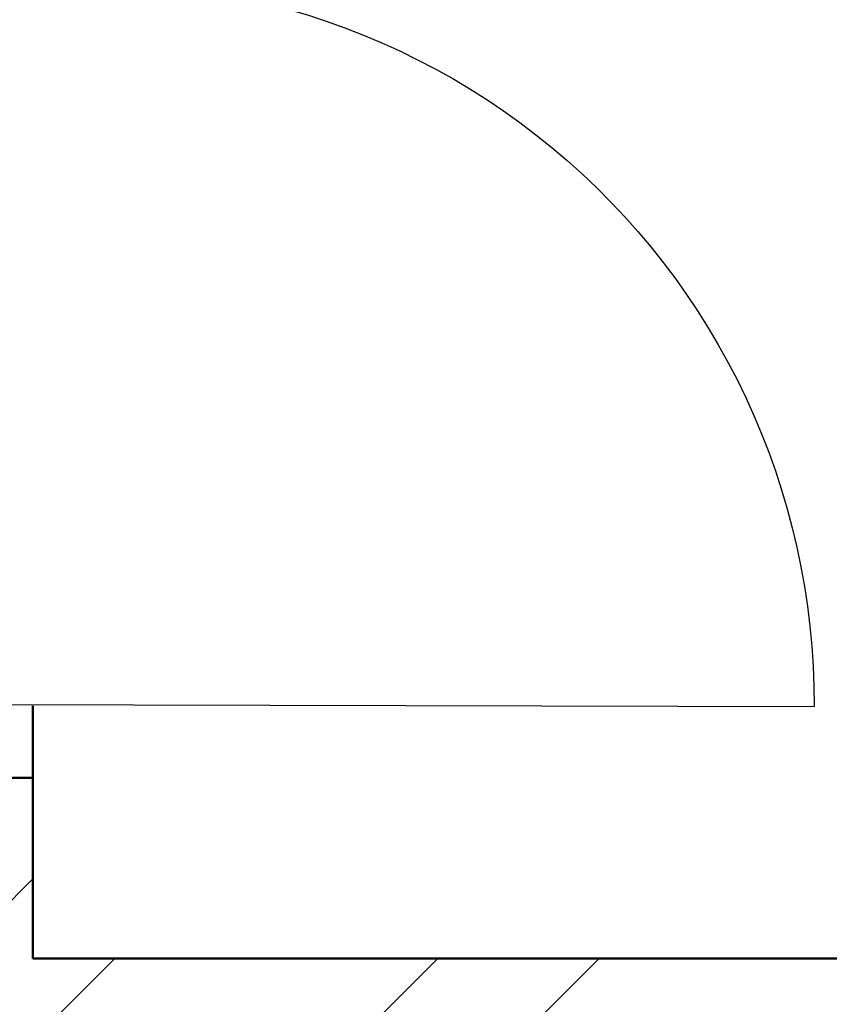
# Model space of a CAD drawing. Units: inches. Extents: x 1901 to 2863, y 888 to 2433.
# Tile 81 of 91: x 2659 to 2682, y 2009 to 2037. Entities that reach past the tile are written whole.
import ezdxf

# ---------------------------------------------------------------- set-up
doc = ezdxf.new("R2010")
doc.units = ezdxf.units.IN
for name, color, linetype, lineweight in [('A-DOOR', 4, 'Continuous', 25), ('A-WALL', 7, 'Continuous', 50), ('A-WALL-PATT', 8, 'Continuous', 13)]:
    doc.layers.add(name, color=color, linetype=linetype, lineweight=lineweight)

# ---------------------------------------------------------------- blocks, each defined once
blk = doc.blocks.new('DOOR-20B')
blk.add_line((0.002, -0.016), (0.002, 23.984))
blk.add_arc((0.002, 3.902), 20.082, 348.7487, 90)

msp = doc.modelspace()

# ---------------------------------------------------------------- hatches: boundary and pattern name
at = {"layer": 'A-WALL-PATT'}
h = msp.add_hatch(dxfattribs=at)
h.set_pattern_fill('ANSI32', color=256)
h.paths.add_polyline_path([(2192.501, 2274.134), (2141.264, 2274.134), (2141.264, 2269.634), (2192.501, 2269.634)])
h.paths.add_polyline_path([(2259.926, 2274.134), (2216.501, 2274.134), (2216.501, 2269.634), (2255.426, 2269.634), (2255.426, 2214.634), (2250.809, 2214.634), (2250.809, 2210.134), (2259.926, 2210.134), (2259.926, 2215.134), (2271.756, 2215.134), (2271.756, 2217.384), (2271.756, 2219.634), (2259.926, 2219.634)])
h.paths.add_polyline_path([(2171.426, 2269.634), (2166.926, 2269.634), (2166.926, 2219.634), (2121.238, 2219.634), (2121.238, 2215.134), (2166.926, 2215.134), (2166.926, 2083.134), (2161.807, 2083.134), (2161.807, 2078.634), (2171.426, 2078.634), (2176.996, 2078.634), (2176.996, 2080.884), (2176.996, 2083.134), (2171.426, 2083.134), (2171.426, 2210.134), (2230.912, 2210.134), (2230.912, 2212.384), (2230.912, 2214.634), (2171.426, 2214.634)])
h.paths.add_polyline_path([(2117.264, 2274.134), (2089.426, 2274.134), (2089.426, 2219.634), (2081.136, 2219.634), (2081.136, 2215.134), (2089.426, 2215.134), (2098.004, 2215.134), (2098.004, 2217.384), (2098.004, 2219.634), (2093.926, 2219.634), (2093.926, 2269.634), (2117.264, 2269.634), (2117.264, 2271.884)])
h.paths.add_polyline_path([(2343.426, 2219.634), (2329.295, 2219.634), (2329.295, 2215.134), (2338.926, 2215.134), (2338.926, 2184.739), (2343.426, 2184.739)])
h.paths.add_polyline_path([(2338.926, 2083.134), (2329.295, 2083.134), (2208.966, 2083.134), (2208.966, 2078.634), (2338.926, 2078.634)])
h.paths.add_polyline_path([(2343.426, 2136.739), (2338.926, 2136.739), (2338.926, 1872.634), (2343.426, 1872.634)])
h.paths.add_polyline_path([(2343.426, 1863.634), (2397.68, 1863.634), (2397.68, 1821.634), (2384.138, 1821.634), (2384.138, 1812.634), (2418.33, 1812.634), (2418.33, 1817.134), (2418.33, 1821.634), (2406.68, 1821.634), (2406.68, 1863.634), (2459.499, 1863.634), (2459.499, 1821.634), (2447.138, 1821.634), (2447.138, 1812.634), (2459.499, 1812.634), (2468.499, 1812.634), (2468.499, 1872.634), (2394.426, 1872.634), (2334.426, 1872.634), (2334.426, 1812.634), (2343.426, 1812.634), (2353.251, 1812.634), (2353.251, 1821.634), (2343.426, 1821.634)])
h.paths.add_polyline_path([(2510.014, 1872.634), (2468.499, 1872.634), (2468.499, 1868.134), (2510.014, 1868.134)])
h.paths.add_polyline_path([(2514.009, 1817.134), (2468.499, 1817.134), (2468.499, 1812.634), (2482.114, 1812.634), (2482.114, 1800.606), (2486.614, 1800.606), (2486.614, 1812.634), (2514.009, 1812.634)])
h.paths.add_polyline_path([(2299.247, 1814.884), (2299.247, 1817.134), (2295.926, 1817.134), (2295.926, 1854.169), (2293.676, 1854.169), (2291.426, 1854.169), (2291.426, 1817.134), (2266.109, 1817.134), (2266.109, 1812.634), (2299.247, 1812.634)])
h.paths.add_polyline_path([(2218.109, 1817.134), (2206.46, 1817.134), (2171.426, 1817.134), (2171.426, 1949.134), (2190.1, 1949.134), (2190.1, 1953.634), (2163.468, 1953.634), (2163.468, 1949.134), (2166.926, 1949.134), (2166.926, 1817.134), (2114.297, 1817.134), (2114.297, 1812.634), (2218.109, 1812.634)])
h.paths.add_polyline_path([(2029.426, 1970.922), (2024.926, 1970.922), (2024.926, 1912.717), (2029.426, 1912.717)])
h.paths.add_polyline_path([(2132.297, 1953.634), (2113.926, 1953.634), (2113.926, 1975.888), (2111.676, 1975.888), (2109.426, 1975.888), (2109.426, 1953.634), (2029.426, 1953.634), (2029.426, 1949.134), (2132.297, 1949.134)])
h.paths.add_polyline_path([(2029.426, 1853.606), (2029.31, 1853.606), (2029.31, 1853.606), (2029.426, 1853.606), (2029.426, 1864.717), (2024.926, 1864.717), (2024.926, 1812.634), (2066.297, 1812.634), (2066.297, 1814.884), (2066.297, 1817.134), (2029.426, 1817.134)])
h.paths.add_polyline_path([(2122.926, 2010.088), (2120.676, 2010.088), (2118.426, 2010.088), (2118.426, 2006.134), (2029.426, 2006.134), (2029.426, 2001.634), (2109.426, 2001.634), (2109.426, 1998.041), (2113.926, 1998.041), (2113.926, 2001.634), (2122.926, 2001.634)])
h.paths.add_polyline_path([(2029.426, 2031.376), (2024.926, 2031.376), (2024.926, 1994.922), (2027.176, 1994.922), (2029.426, 1994.922)])
h.paths.add_polyline_path([(2029.426, 2136.739), (2024.926, 2136.739), (2024.926, 2067.376), (2027.176, 2067.376), (2029.426, 2067.376)])
h.paths.add_polyline_path([(2125.618, 2083.134), (2029.426, 2083.134), (2029.426, 2078.634), (2118.426, 2078.634), (2118.426, 2030.715), (2122.926, 2030.715), (2122.926, 2078.634), (2125.618, 2078.634)])
h.paths.add_polyline_path([(2029.426, 2215.134), (2040.468, 2215.134), (2040.468, 2217.384), (2040.468, 2219.634), (2024.926, 2219.634), (2024.926, 2184.739), (2029.426, 2184.739), (2029.426, 2187.778)])
h.paths.add_polyline_path([(2686.426, 2274.134), (2659.284, 2274.134), (2659.284, 2269.634), (2681.926, 2269.634), (2681.926, 2219.634), (2676.816, 2219.634), (2676.816, 2215.134), (2681.926, 2215.134), (2697.011, 2215.134), (2697.011, 2217.384), (2697.011, 2219.634), (2686.426, 2219.634)])
h.paths.add_polyline_path([(2609.926, 2269.634), (2635.284, 2269.634), (2635.284, 2274.134), (2571.431, 2274.134), (2571.431, 2269.634), (2605.426, 2269.634), (2605.426, 2214.634), (2549.098, 2214.634), (2549.098, 2210.134), (2605.426, 2210.134), (2605.426, 2083.134), (2601.014, 2083.134), (2601.014, 2080.884), (2601.014, 2078.634), (2609.926, 2078.634), (2616.162, 2078.634), (2616.162, 2080.884), (2616.162, 2083.134), (2609.926, 2083.134), (2609.926, 2215.134), (2651.465, 2215.134), (2651.465, 2217.384), (2651.465, 2219.634), (2609.926, 2219.634)])
h.paths.add_polyline_path([(2521.426, 2269.634), (2547.431, 2269.634), (2547.431, 2271.884), (2547.431, 2274.134), (2516.926, 2274.134), (2516.926, 2219.634), (2506.41, 2219.634), (2506.41, 2215.134), (2516.926, 2215.134), (2516.926, 2210.134), (2525.402, 2210.134), (2525.402, 2212.384), (2525.402, 2214.634), (2521.426, 2214.634)])
h.paths.add_polyline_path([(2456.011, 2219.634), (2439.426, 2219.634), (2439.426, 2187.888), (2443.926, 2187.888), (2443.926, 2215.134), (2456.011, 2215.134)])
h.paths.add_polyline_path([(2752.926, 2219.634), (2739.485, 2219.634), (2739.485, 2215.134), (2748.426, 2215.134), (2748.426, 2187.888), (2752.926, 2187.888)])
h.paths.add_polyline_path([(2752.926, 2139.888), (2748.426, 2139.888), (2748.426, 2083.134), (2648.416, 2083.134), (2648.416, 2078.634), (2654.926, 2078.634), (2654.926, 2039.437), (2659.426, 2039.437), (2659.426, 2078.634), (2748.426, 2078.634), (2748.426, 2063.429), (2752.926, 2063.429)])
h.paths.add_polyline_path([(2752.926, 2010.634), (2659.426, 2010.634), (2659.426, 2015.652), (2654.926, 2015.652), (2654.926, 2010.634), (2605.426, 2010.634), (2605.426, 1920.967), (2609.926, 1920.967), (2609.926, 2006.134), (2748.426, 2006.134), (2748.426, 1982.466), (2752.926, 1982.466)])
h.paths.add_polyline_path([(2752.926, 2027.429), (2748.426, 2027.429), (2748.426, 2010.634), (2752.926, 2010.634)])
h.paths.add_polyline_path([(2748.426, 1886.134), (2609.926, 1886.134), (2609.926, 1889.719), (2605.426, 1889.719), (2605.426, 1861.262), (2609.926, 1861.262), (2609.926, 1881.634), (2748.426, 1881.634)])
h.paths.add_polyline_path([(2456.855, 2228.831), (2498.401, 2228.831), (2498.401, 2247.488), (2456.855, 2247.488)], flags=9)
h.paths.add_polyline_path([(2038.602, 2237.418), (2080.174, 2237.418), (2080.174, 2256.075), (2038.602, 2256.075)], flags=9)
h.paths.add_polyline_path([(2292.009, 1062.394), (2539.932, 1062.394), (2539.932, 1099.487), (2292.009, 1099.487)], flags=9)
h.paths.add_polyline_path([(2424.91, 1832.253), (2448.513, 1832.253), (2448.513, 1846.678), (2424.91, 1846.678)], flags=25)
h.paths.add_polyline_path([(2359.076, 1832.253), (2382.678, 1832.253), (2382.678, 1846.678), (2359.076, 1846.678)], flags=25)
h.paths.add_polyline_path([(2352.899, 1684.802), (2367.543, 1684.802), (2367.543, 1697.167), (2352.899, 1697.167)], flags=9)
h.paths.add_polyline_path([(2079.288, 1755.826), (2169.024, 1755.826), (2169.024, 1774.372), (2079.288, 1774.372)], flags=9)
h.paths.add_polyline_path([(2404.09, 1373.857), (2404.09, 1463.593), (2385.544, 1463.593), (2385.544, 1373.857)], flags=9)
h.paths.add_polyline_path([(2268.091, 2236.371), (2309.636, 2236.371), (2309.636, 2255.028), (2268.091, 2255.028)], flags=9)
h.paths.add_polyline_path([(2575.96, 1700.951), (2665.696, 1700.951), (2665.696, 1719.498), (2575.96, 1719.498)], flags=9)
h.paths.add_polyline_path([(2302.962, 1878.474), (2329.524, 1878.474), (2329.524, 1888.777), (2302.962, 1888.777)], flags=9)
h.paths.add_polyline_path([(2097.415, 2240.576), (2126.573, 2240.576), (2126.573, 2259.233), (2097.415, 2259.233)], flags=9)
h.paths.add_polyline_path([(2208.725, 2246.124), (2237.882, 2246.124), (2237.882, 2264.781), (2208.725, 2264.781)], flags=9)
h.paths.add_polyline_path([(2038.147, 1925.958), (2076.987, 1925.958), (2076.987, 1944.615), (2038.147, 1944.615)], flags=9)
h.paths.add_polyline_path([(2239.144, 1926.672), (2288.465, 1926.672), (2288.465, 1945.329), (2239.144, 1945.329)], flags=9)
h.paths.add_polyline_path([(2175.429, 2007.33), (2212.356, 2007.33), (2212.356, 2025.987), (2175.429, 2025.987)], flags=9)
h.paths.add_polyline_path([(2225.034, 2091.794), (2263.875, 2091.794), (2263.875, 2110.451), (2225.034, 2110.451)], flags=9)
h.paths.add_polyline_path([(2035.398, 2098.478), (2074.238, 2098.478), (2074.238, 2117.135), (2035.398, 2117.135)], flags=9)
h.paths.add_polyline_path([(2050.102, 2029.209), (2083.26, 2029.209), (2083.26, 2047.866), (2050.102, 2047.866)], flags=9)
h.paths.add_polyline_path([(2069.677, 1956.719), (2098.835, 1956.719), (2098.835, 1975.376), (2069.677, 1975.376)], flags=25)
h.paths.add_polyline_path([(2328.62, 1753.336), (2361.663, 1753.336), (2361.663, 1771.993), (2328.62, 1771.993)], flags=9)
h.paths.add_polyline_path([(2395.162, 2060.888), (2395.162, 2140.654), (2378.676, 2140.654), (2378.676, 2060.888)], flags=9)
h.paths.add_polyline_path([(2463.728, 2059.02), (2492.886, 2059.02), (2492.886, 2077.677), (2463.728, 2077.677)], flags=9)
h.paths.add_polyline_path([(2458.027, 2181.536), (2496.868, 2181.536), (2496.868, 2200.194), (2458.027, 2200.194)], flags=9)
h.paths.add_polyline_path([(2527.577, 2243.074), (2556.735, 2243.074), (2556.735, 2261.731), (2527.577, 2261.731)], flags=9)
h.paths.add_polyline_path([(2694.461, 2232.767), (2736.033, 2232.767), (2736.033, 2251.425), (2694.461, 2251.425)], flags=9)
h.paths.add_polyline_path([(2637.821, 2249.225), (2666.979, 2249.225), (2666.979, 2267.882), (2637.821, 2267.882)], flags=9)
h.paths.add_polyline_path([(2623.687, 2183.541), (2662.528, 2183.541), (2662.528, 2202.199), (2623.687, 2202.199)], flags=9)
h.paths.add_polyline_path([(2691.965, 2021.5), (2725.124, 2021.5), (2725.124, 2040.157), (2691.965, 2040.157)], flags=9)
h.paths.add_polyline_path([(2621.043, 1975.912), (2662.335, 1975.912), (2662.335, 1994.569), (2621.043, 1994.569)], flags=25)
h.paths.add_polyline_path([(2479.032, 1927.62), (2519.844, 1927.62), (2519.844, 1946.277), (2479.032, 1946.277)], flags=9)
h.paths.add_polyline_path([(2670.941, 1849.076), (2716.005, 1849.076), (2716.005, 1867.734), (2670.941, 1867.734)], flags=9)
h.paths.add_polyline_path([(2523.613, 1782.956), (2550.175, 1782.956), (2550.175, 1793.26), (2523.613, 1793.26)], flags=9)
h.paths.add_polyline_path([(2450.841, 1207.331), (2492.386, 1207.331), (2492.386, 1225.989), (2450.841, 1225.989)], flags=9)
h.paths.add_polyline_path([(2527.751, 1203.841), (2556.908, 1203.841), (2556.908, 1222.499), (2527.751, 1222.499)], flags=9)
h.paths.add_polyline_path([(2639.111, 1207.2), (2668.268, 1207.2), (2668.268, 1225.857), (2639.111, 1225.857)], flags=9)
h.paths.add_polyline_path([(2692.594, 1218.965), (2734.167, 1218.965), (2734.167, 1237.623), (2692.594, 1237.623)], flags=9)
h.paths.add_polyline_path([(2669.266, 1366.329), (2708.106, 1366.329), (2708.106, 1384.987), (2669.266, 1384.987)], flags=9)
h.paths.add_polyline_path([(2463.313, 1358.031), (2502.153, 1358.031), (2502.153, 1376.688), (2463.313, 1376.688)], flags=9)
h.paths.add_polyline_path([(2494.725, 1449.963), (2531.652, 1449.963), (2531.652, 1468.62), (2494.725, 1468.62)], flags=9)
h.paths.add_polyline_path([(2675.565, 1422.157), (2708.724, 1422.157), (2708.724, 1440.815), (2675.565, 1440.815)], flags=9)
h.paths.add_polyline_path([(2685.634, 1493.891), (2714.792, 1493.891), (2714.792, 1512.548), (2685.634, 1512.548)], flags=9)
h.paths.add_polyline_path([(2686.805, 1529.913), (2725.645, 1529.913), (2725.645, 1548.57), (2686.805, 1548.57)], flags=9)
h.paths.add_polyline_path([(2503.651, 1537.991), (2552.972, 1537.991), (2552.972, 1556.648), (2503.651, 1556.648)], flags=9)
h.paths.add_polyline_path([(2291.713, 1643.504), (2318.275, 1643.504), (2318.275, 1653.807), (2291.713, 1653.807)], flags=9)
h.paths.add_polyline_path([(2450.626, 1610.52), (2477.189, 1610.52), (2477.189, 1620.824), (2450.626, 1620.824)], flags=9)
h.paths.add_polyline_path([(2359.985, 1551.814), (2422.253, 1551.814), (2422.253, 1562.117), (2359.985, 1562.117)], flags=9)
h.paths.add_polyline_path([(2280.106, 1249.006), (2321.651, 1249.006), (2321.651, 1267.663), (2280.106, 1267.663)], flags=9)
h.paths.add_polyline_path([(2164.057, 1274.232), (2193.215, 1274.232), (2193.215, 1292.889), (2164.057, 1292.889)], flags=9)
h.paths.add_polyline_path([(2118.21, 1277.694), (2151.252, 1277.694), (2151.252, 1296.351), (2118.21, 1296.351)], flags=9)
h.paths.add_polyline_path([(2031.946, 1268.529), (2073.519, 1268.529), (2073.519, 1287.187), (2031.946, 1287.187)], flags=9)
h.paths.add_polyline_path([(2050.199, 1409.079), (2089.04, 1409.079), (2089.04, 1427.736), (2050.199, 1427.736)], flags=9)
h.paths.add_polyline_path([(2243.743, 1421.032), (2282.584, 1421.032), (2282.584, 1439.689), (2243.743, 1439.689)], flags=9)
h.paths.add_polyline_path([(2190.746, 1509.769), (2231.558, 1509.769), (2231.558, 1528.426), (2190.746, 1528.426)], flags=9)
h.paths.add_polyline_path([(2058.392, 1475.415), (2091.55, 1475.415), (2091.55, 1494.073), (2058.392, 1494.073)], flags=9)
h.paths.add_polyline_path([(2062.447, 1553.09), (2091.605, 1553.09), (2091.605, 1571.747), (2062.447, 1571.747)], flags=9)
h.paths.add_polyline_path([(2219.524, 1590.365), (2266.147, 1590.365), (2266.147, 1609.022), (2219.524, 1609.022)], flags=9)
h.paths.add_polyline_path([(2041.072, 1584.188), (2079.912, 1584.188), (2079.912, 1602.845), (2041.072, 1602.845)], flags=9)

# ---------------------------------------------------------------- linework, layer by layer
at = {"layer": 'A-WALL'}
for p, q in [((2659.426, 2010.634), (2659.426, 2017.652)), ((2659.426, 2015.652), (2654.926, 2015.652)), ((2659.426, 2010.634), (2748.426, 2010.634)), ((2752.926, 2010.634), (2659.426, 2010.634))]:
    msp.add_line(p, q, dxfattribs=at)

# ---------------------------------------------------------------- block references
at = {"layer": 'A-DOOR', "extrusion": (0, 0, -1), "zscale": -1, "rotation": 90.1553947244059}
msp.add_blockref('DOOR-20B', (-2657.167, 2017.696), dxfattribs=at)

doc.saveas('drawing.dxf')
